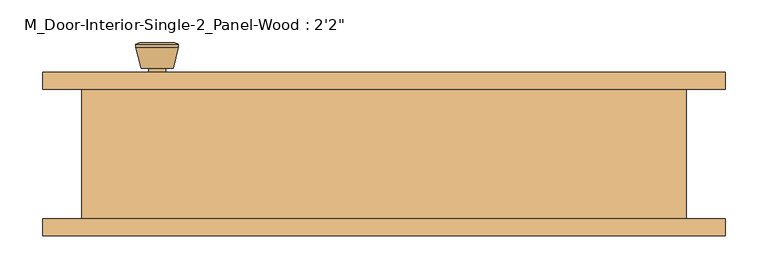
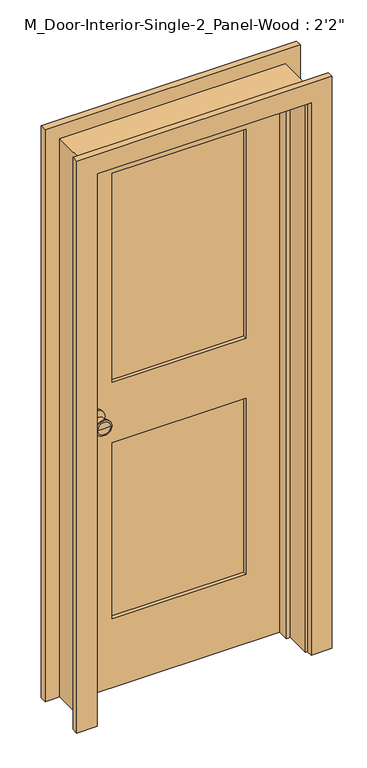
"""IFC4 building model written with IfcOpenShell, lengths in millimetres: door geometry."""

from ifc_helpers import new_model, si_unit, point, frame, frame_2d, origin, place, context, project, spatial, polyline, circle_curve, trimmed, segment, composite_curve, outline, extrude, faceted_brep, source, transform, mapped, element, save
from ifc_brep_helpers import plane_surface, cylinder_surface, revolved_surface, advanced_brep


def door_57d9c04c(model_context):
    return source(origin(), model_context, "Body", "SolidModel", [
        advanced_brep(
        [(-266.7, 32.025, 914.4), (-256.7, 32.025, 914.4), (-276.7, 32.025, 914.4), (-246.2241324, -16.975, 914.4), (-266.7, -16.975, 914.4), (-287.1758676, -16.975, 914.4), (-241.7, -15.1471319, 914.4), (-291.7, -15.1471319, 914.4), (-241.7, -11.6834537, 914.4), (-291.7, -11.6834537, 914.4), (-248.063764, 13.025, 914.4), (-285.336236, 13.025, 914.4), (-256.7, 13.025, 914.4), (-276.7, 13.025, 914.4)],
        [
            (0, 1),
            (1, 2, circle_curve(frame((-266.7, 32.025, 914.4), z_axis=(0.0, 1.0, 0.0), x_axis=(-1.0, 0.0, 0.0)), 10.0)),
            (2, 0),
            (2, 1, circle_curve(frame((-266.7, 32.025, 914.4), z_axis=(0.0, 1.0, 0.0), x_axis=(-1.0, 0.0, 0.0)), 10.0)),
            (3, 4),
            (4, 5),
            (5, 3, circle_curve(frame((-266.7, -16.975, 914.4), z_axis=(0.0, -1.0, 0.0), x_axis=(-1.0, 0.0, 0.0)), 20.4758676)),
            (3, 5, circle_curve(frame((-266.7, -16.975, 914.4), z_axis=(0.0, -1.0, 0.0), x_axis=(-1.0, 0.0, 0.0)), 20.4758676)),
            (6, 3),
            (5, 7),
            (7, 6, circle_curve(frame((-266.7, -15.1471319, 914.4), z_axis=(0.0, -1.0, 0.0), x_axis=(-1.0, 0.0, 0.0)), 25.0)),
            (6, 7, circle_curve(frame((-266.7, -15.1471319, 914.4), z_axis=(0.0, -1.0, 0.0), x_axis=(-1.0, 0.0, 0.0)), 25.0)),
            (8, 6),
            (7, 9),
            (9, 8, circle_curve(frame((-266.7, -11.6834537, 914.4), z_axis=(0.0, -1.0, 0.0), x_axis=(-1.0, 0.0, 0.0)), 25.0)),
            (8, 9, circle_curve(frame((-266.7, -11.6834537, 914.4), z_axis=(0.0, -1.0, 0.0), x_axis=(-1.0, 0.0, 0.0)), 25.0)),
            (10, 8),
            (9, 11),
            (11, 10, circle_curve(frame((-266.7, 13.025, 914.4), z_axis=(0.0, -1.0, 0.0), x_axis=(-1.0, 0.0, 0.0)), 18.636236)),
            (10, 11, circle_curve(frame((-266.7, 13.025, 914.4), z_axis=(0.0, -1.0, 0.0), x_axis=(-1.0, 0.0, 0.0)), 18.636236)),
            (12, 10),
            (11, 13),
            (13, 12, circle_curve(frame((-266.7, 13.025, 914.4), z_axis=(0.0, -1.0, 0.0), x_axis=(-1.0, 0.0, 0.0)), 10.0)),
            (12, 13, circle_curve(frame((-266.7, 13.025, 914.4), z_axis=(0.0, -1.0, 0.0), x_axis=(-1.0, 0.0, 0.0)), 10.0)),
            (1, 12),
            (13, 2),
        ],
        [
            plane_surface(frame((-266.7, 32.025, 914.4), z_axis=(0.0, 1.0, 0.0), x_axis=(-1.0, 0.0, 0.0))),
            plane_surface(frame((-266.7, -16.975, 914.4), z_axis=(0.0, -1.0, 0.0), x_axis=(-1.0, 0.0, 0.0))),
            revolved_surface(polyline([(-287.1758676, -16.975, 914.4), (-291.7, -15.1471319, 914.4)]), (-266.7, 32.025, 914.4), (0.0, 1.0, 0.0)),
            cylinder_surface(frame((-266.7, 32.025, 914.4), z_axis=(0.0, 1.0, 0.0), x_axis=(-1.0, 0.0, 0.0)), 25.0),
            revolved_surface(polyline([(-291.7, -11.6834537, 914.4), (-285.336236, 13.025, 914.4)]), (-266.7, 32.025, 914.4), (0.0, 1.0, 0.0)),
            plane_surface(frame((-266.7, 13.025, 914.4), z_axis=(0.0, 1.0, 0.0), x_axis=(-1.0, 0.0, 0.0))),
            cylinder_surface(frame((-266.7, 32.025, 914.4), z_axis=(0.0, 1.0, 0.0), x_axis=(-1.0, 0.0, 0.0)), 10.0),
        ],
        [
            (0, [[1, 2, 3]]),
            (0, [[-3, 4, -1]]),
            (1, [[5, 6, 7]]),
            (1, [[-6, -5, 8]]),
            (2, [[9, -7, 10, 11]]),
            (2, [[-10, -8, -9, 12]]),
            (3, [[13, -11, 14, 15]]),
            (3, [[-14, -12, -13, 16]]),
            (4, [[17, -15, 18, 19]]),
            (4, [[-18, -16, -17, 20]]),
            (5, [[21, -19, 22, 23]]),
            (5, [[-22, -20, -21, 24]]),
            (6, [[25, -23, 26, -2]]),
            (6, [[-26, -24, -25, -4]]),
        ],
    ),
        extrude(outline(composite_curve([segment(trimmed(circle_curve(frame_2d((914.4, -266.7)), 30.0), [point((914.4, -296.7))], [point((914.4, -236.7))], False, "CARTESIAN"), True, "CONTINUOUS"), segment(trimmed(circle_curve(frame_2d((914.4, -266.7)), 30.0), [point((914.4, -236.7))], [point((914.4, -296.7))], False, "CARTESIAN"), True, "CONTINUOUS")], self_intersect=False)), frame((0.0, 32.025, 0.0), z_axis=(0.0, 1.0, 0.0), x_axis=(0.0, 0.0, 1.0)), (0.0, 0.0, 1.0), 6.0),
        advanced_brep(
        [(-266.7, 79.025, 914.4), (-276.7, 79.025, 914.4), (-256.7, 79.025, 914.4), (-246.2241324, 128.025, 914.4), (-287.1758676, 128.025, 914.4), (-266.7, 128.025, 914.4), (-241.7, 126.1971319, 914.4), (-291.7, 126.1971319, 914.4), (-241.7, 122.7334537, 914.4), (-291.7, 122.7334537, 914.4), (-248.063764, 98.025, 914.4), (-285.336236, 98.025, 914.4), (-256.7, 98.025, 914.4), (-276.7, 98.025, 914.4)],
        [
            (0, 1),
            (1, 2, circle_curve(frame((-266.7, 79.025, 914.4), z_axis=(0.0, -1.0, 0.0), x_axis=(-1.0, 0.0, 0.0)), 10.0)),
            (2, 0),
            (2, 1, circle_curve(frame((-266.7, 79.025, 914.4), z_axis=(0.0, -1.0, 0.0), x_axis=(-1.0, 0.0, 0.0)), 10.0)),
            (3, 4, circle_curve(frame((-266.7, 128.025, 914.4), z_axis=(0.0, 1.0, 0.0), x_axis=(-1.0, 0.0, 0.0)), 20.4758676)),
            (4, 5),
            (5, 3),
            (4, 3, circle_curve(frame((-266.7, 128.025, 914.4), z_axis=(0.0, 1.0, 0.0), x_axis=(-1.0, 0.0, 0.0)), 20.4758676)),
            (6, 7, circle_curve(frame((-266.7, 126.1971319, 914.4), z_axis=(0.0, 1.0, 0.0), x_axis=(-1.0, 0.0, 0.0)), 25.0)),
            (7, 4),
            (3, 6),
            (7, 6, circle_curve(frame((-266.7, 126.1971319, 914.4), z_axis=(0.0, 1.0, 0.0), x_axis=(-1.0, 0.0, 0.0)), 25.0)),
            (8, 9, circle_curve(frame((-266.7, 122.7334537, 914.4), z_axis=(0.0, 1.0, 0.0), x_axis=(-1.0, 0.0, 0.0)), 25.0)),
            (9, 7),
            (6, 8),
            (9, 8, circle_curve(frame((-266.7, 122.7334537, 914.4), z_axis=(0.0, 1.0, 0.0), x_axis=(-1.0, 0.0, 0.0)), 25.0)),
            (10, 11, circle_curve(frame((-266.7, 98.025, 914.4), z_axis=(0.0, 1.0, 0.0), x_axis=(-1.0, 0.0, 0.0)), 18.636236)),
            (11, 9),
            (8, 10),
            (11, 10, circle_curve(frame((-266.7, 98.025, 914.4), z_axis=(0.0, 1.0, 0.0), x_axis=(-1.0, 0.0, 0.0)), 18.636236)),
            (12, 13, circle_curve(frame((-266.7, 98.025, 914.4), z_axis=(0.0, 1.0, 0.0), x_axis=(-1.0, 0.0, 0.0)), 10.0)),
            (13, 11),
            (10, 12),
            (13, 12, circle_curve(frame((-266.7, 98.025, 914.4), z_axis=(0.0, 1.0, 0.0), x_axis=(-1.0, 0.0, 0.0)), 10.0)),
            (1, 13),
            (12, 2),
        ],
        [
            plane_surface(frame((-266.7, 79.025, 914.4), z_axis=(0.0, -1.0, 0.0), x_axis=(-1.0, 0.0, 0.0))),
            plane_surface(frame((-266.7, 128.025, 914.4), z_axis=(0.0, 1.0, 0.0), x_axis=(-1.0, 0.0, 0.0))),
            revolved_surface(polyline([(-287.1758676, 128.025, 914.4), (-291.7, 126.1971319, 914.4)]), (-266.7, 79.025, 914.4), (0.0, -1.0, 0.0)),
            cylinder_surface(frame((-266.7, 79.025, 914.4), z_axis=(0.0, -1.0, 0.0), x_axis=(-1.0, 0.0, 0.0)), 25.0),
            revolved_surface(polyline([(-291.7, 122.7334537, 914.4), (-285.336236, 98.025, 914.4)]), (-266.7, 79.025, 914.4), (0.0, -1.0, 0.0)),
            plane_surface(frame((-266.7, 98.025, 914.4), z_axis=(0.0, -1.0, 0.0), x_axis=(-1.0, 0.0, 0.0))),
            cylinder_surface(frame((-266.7, 79.025, 914.4), z_axis=(0.0, -1.0, 0.0), x_axis=(-1.0, 0.0, 0.0)), 10.0),
        ],
        [
            (0, [[1, 2, 3]]),
            (0, [[-3, 4, -1]]),
            (1, [[5, 6, 7]]),
            (1, [[8, -7, -6]]),
            (2, [[9, 10, -5, 11]]),
            (2, [[12, -11, -8, -10]]),
            (3, [[13, 14, -9, 15]]),
            (3, [[16, -15, -12, -14]]),
            (4, [[17, 18, -13, 19]]),
            (4, [[20, -19, -16, -18]]),
            (5, [[21, 22, -17, 23]]),
            (5, [[24, -23, -20, -22]]),
            (6, [[-2, 25, -21, 26]]),
            (6, [[-4, -26, -24, -25]]),
        ],
    ),
        extrude(outline(composite_curve([segment(trimmed(circle_curve(frame_2d((914.4, -266.7)), 30.0), [point((914.4, -296.7))], [point((914.4, -236.7))], False, "CARTESIAN"), True, "CONTINUOUS"), segment(trimmed(circle_curve(frame_2d((914.4, -266.7)), 30.0), [point((914.4, -236.7))], [point((914.4, -296.7))], False, "CARTESIAN"), True, "CONTINUOUS")], self_intersect=False)), frame((0.0, 73.025, 0.0), z_axis=(0.0, 1.0, 0.0), x_axis=(0.0, 0.0, 1.0)), (0.0, 0.0, 1.0), 6.0),
        faceted_brep([(355.2, 73.025, 0.0), (355.2, -79.375, 0.0), (330.2, -79.375, 0.0), (330.2, 3.1, 0.0), (317.5, 3.1, 0.0), (317.5, 38.025, 0.0), (330.2, 38.025, 0.0), (330.2, 73.025, 0.0), (355.2, 73.025, 1853.8), (355.2, -79.375, 1853.8), (-355.2, -79.375, 1853.8), (-355.2, -79.375, 0.0), (-330.2, -79.375, 0.0), (-330.2, -79.375, 1828.8), (330.2, -79.375, 1828.8), (330.2, 3.1, 1828.8), (-330.2, 3.1, 1828.8), (-330.2, 3.1, 0.0), (-317.5, 3.1, 0.0), (-317.5, 3.1, 1816.1), (317.5, 3.1, 1816.1), (317.5, 38.025, 1816.1), (-317.5, 38.025, 1816.1), (-317.5, 38.025, 0.0), (-330.2, 38.025, 0.0), (-330.2, 38.025, 1828.8), (330.2, 38.025, 1828.8), (330.2, 73.025, 1828.8), (-330.2, 73.025, 1828.8), (-330.2, 73.025, 0.0), (-355.2, 73.025, 0.0), (-355.2, 73.025, 1853.8)], [[[0, 1, 2, 3, 4, 5, 6, 7]], [[1, 0, 8, 9]], [[2, 1, 9, 10, 11, 12, 13, 14]], [[3, 2, 14, 15]], [[4, 3, 15, 16, 17, 18, 19, 20]], [[5, 4, 20, 21]], [[6, 5, 21, 22, 23, 24, 25, 26]], [[7, 6, 26, 27]], [[0, 7, 27, 28, 29, 30, 31, 8]], [[9, 8, 31, 10]], [[15, 14, 13, 16]], [[21, 20, 19, 22]], [[27, 26, 25, 28]], [[30, 29, 24, 23, 18, 17, 12, 11]], [[10, 31, 30, 11]], [[16, 13, 12, 17]], [[22, 19, 18, 23]], [[28, 25, 24, 29]]]),
        extrude(outline(polyline([(1828.8, -330.2), (0.0, -330.2), (0.0, 330.2), (1828.8, 330.2), (1828.8, -330.2)]), holes=[polyline([(1708.8, -210.2), (1708.8, 210.2), (1014.4, 210.2), (1014.4, -210.2), (1708.8, -210.2)]), polyline([(814.4, -210.2), (814.4, 210.2), (230.0, 210.2), (230.0, -210.2), (814.4, -210.2)])]), frame((0.0, 38.025, 0.0), z_axis=(0.0, 1.0, 0.0), x_axis=(0.0, 0.0, 1.0)), (0.0, 0.0, 1.0), 35.0),
        extrude(outline(polyline([(210.2, 49.6916667), (-210.2, 49.6916667), (-210.2, 61.3583333), (210.2, 61.3583333), (210.2, 49.6916667)])), frame((0.0, 0.0, 1014.4), z_axis=(0.0, 0.0, 1.0), x_axis=(1.0, 0.0, 0.0)), (0.0, 0.0, 1.0), 694.4),
        extrude(outline(polyline([(210.2, 49.6916667), (-210.2, 49.6916667), (-210.2, 61.3583333), (210.2, 61.3583333), (210.2, 49.6916667)])), frame((0.0, 0.0, 230.0), z_axis=(0.0, 0.0, 1.0), x_axis=(1.0, 0.0, 0.0)), (0.0, 0.0, 1.0), 584.4),
        extrude(outline(polyline([(0.0, 336.55), (0.0, 401.55), (1900.15, 401.55), (1900.15, -401.55), (0.0, -401.55), (0.0, -336.55), (1835.15, -336.55), (1835.15, 336.55), (0.0, 336.55)])), frame((0.0, 73.025, 0.0), z_axis=(0.0, 1.0, 0.0), x_axis=(0.0, 0.0, 1.0)), (0.0, 0.0, 1.0), 20.0),
        extrude(outline(polyline([(0.0, 336.55), (0.0, 401.55), (1900.15, 401.55), (1900.15, -401.55), (0.0, -401.55), (0.0, -336.55), (1835.15, -336.55), (1835.15, 336.55), (0.0, 336.55)])), frame((0.0, -99.375, 0.0), z_axis=(0.0, 1.0, 0.0), x_axis=(0.0, 0.0, 1.0)), (0.0, 0.0, 1.0), 20.0),
    ])


if __name__ == "__main__":
    model = new_model("IFC4")
    model_context = context("Model", 3, world=origin())
    ifc_project = project(units=[si_unit("LENGTHUNIT", "METRE", prefix="MILLI")], contexts=[model_context])
    site = spatial("IfcSite", under=ifc_project)
    building = spatial("IfcBuilding", under=site)
    placement = place(None, origin())
    door_shape = door_57d9c04c(model_context)
    element("IfcDoor", 1, ObjectType="M_Door-Interior-Single-2_Panel-Wood : 2'2\"", at=placement, inside=building, context=model_context, shape_type="MappedRepresentation", body=[
        mapped(door_shape, transform((0.0, 0.0, 0.0), x_axis=(1.0, 0.0, 0.0), y_axis=(0.0, 1.0, 0.0), z_axis=(0.0, 0.0, 1.0))),
    ])
    save(model, "model.ifc")

# Revit data of these elements
# Type "M_Door-Interior-Single-2_Panel-Wood : 2'2\""
#   Type Mark = "11"
#   Assembly Code = "C1020300"
#   Analytic Construction = "Wooden"
#   Top Rail = 0' - 4.72441"
#   Thickness = 0' - 1.37795"
#   Thermal Resistance (R) = 2.5876 (h·ft²·°F)/BTU
#   Swing Angle [instance default] = 90.00°
#   Stiles = 0' - 4.72441"
#   Rough Width = 2' - 3.9685"
#   Rough Height = 6' - 0.98425"
#   Lock Rail = 0' - 7.87402"
#   Height = 6' - 0"
#   Width = 2' - 2"
#   Heat Transfer Coefficient (U) = 0.3865 BTU/(h·ft²·°F)
#   Bottom Rail = 0' - 9.05512"
#   Trim Material = Cherry
#   Panel Material = Cherry
#   Frame Material = Cherry
#   Door Handle Material = Aluminum
#   Visual Light Transmittance = 0
#   Solar Heat Gain Coefficient = 0
#   Wall Closure = (empty or 0)
#   Function = (empty or 0)
# Element 1 (IfcDoor, "M_Door-Interior-Single-2_Panel-Wood : 2'2\"")
#   Materials on its faces: "Cherry", "Aluminum"
# Materials
#   "Cherry": class "Wood", colour RGB 226 177 128, transparency 0, Description = "Prunus Serotina", Cost = 0
#   "Aluminum": class "Metal", colour RGB 247 247 247, transparency 0, Description = "Aluminum 6061", Cost = 0
